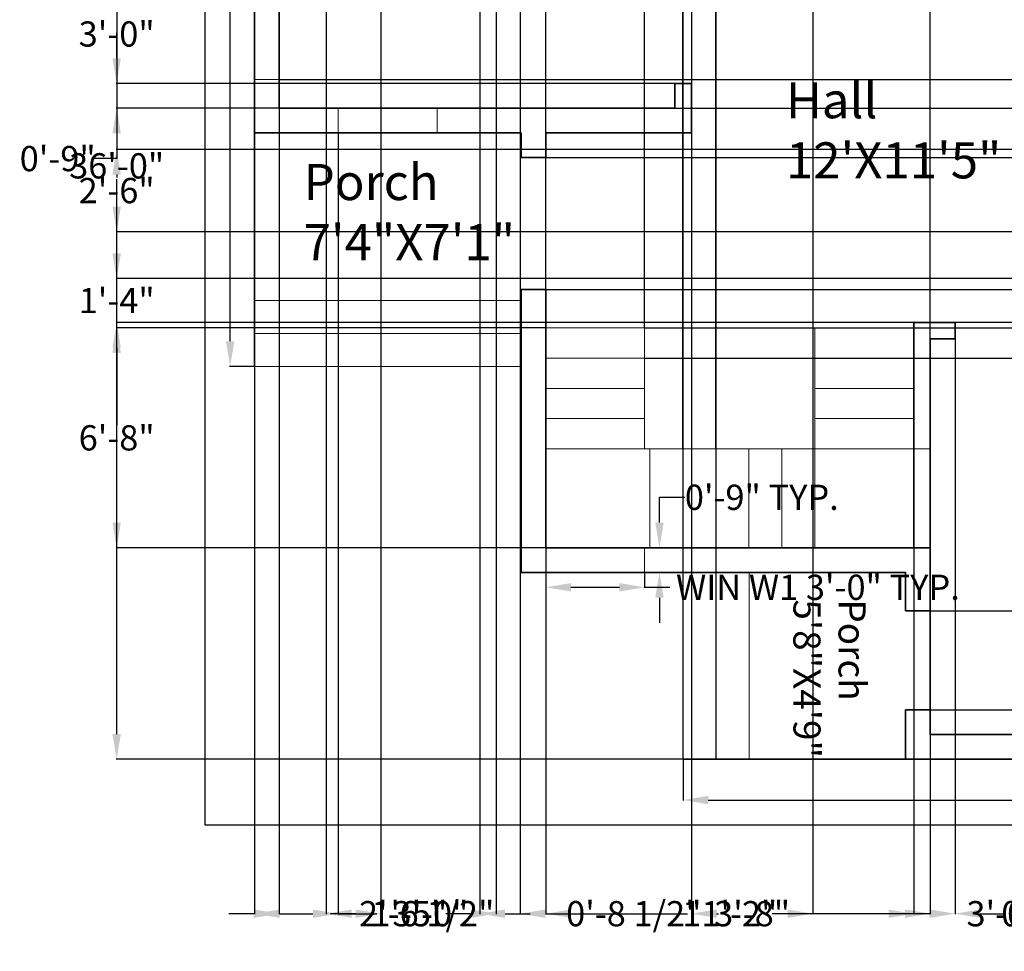
# Model space of a CAD drawing. Units: inches. Extents: x -69 to 558, y -494 to 191.
# Tile 1 of 3: x -69 to 289, y -494 to -155. Entities that reach past the tile are written whole.
import ezdxf

# ---------------------------------------------------------------- set-up
doc = ezdxf.new("R2010")
doc.units = ezdxf.units.IN
doc.header["$MEASUREMENT"] = 0
for name, color, linetype, lineweight in [('A-ANNO-DIMS', 2, 'Continuous', 18), ('A-AREA-IDEN', 7, 'Continuous', 18), ('A-FLOR-STRS', 3, 'Continuous', 18), ('A-GLAZ', 4, 'Continuous', 18), ('A-WALL', 7, 'Continuous', 35), ('C-PROP', 8, 'Continuous', 25)]:
    doc.layers.add(name, color=color, linetype=linetype, lineweight=lineweight)
doc.styles.get("Standard").update_dxf_attribs({"font": 'arial.ttf'})
doc.dimstyles.get("Standard").update_dxf_attribs({"dimtxt": 9.18, "dimasz": 9.18, "dimexe": 0.18, "dimexo": 0.0625, "dimgap": 0.09, "dimtad": 0, "dimtih": 1, "dimtoh": 1, "dimdec": 1, "dimzin": 0, "dimdsep": 46, "dimlunit": 3, "dimtxsty": 'Standard', "dimcen": 9, "dimadec": 0, "dimazin": 0, "dimtfac": 1, "dimtdec": 1, "dimtofl": 0, "dimtmove": 0, "dimatfit": 3, "dimfxl": 1, "dimtolj": 1, "dimtzin": 0, "dimarcsym": 0})

# ---------------------------------------------------------------- blocks, each defined once
blk = doc.blocks.new('*U1')
blk.add_line((-18, 0), (18, 0))
blk = doc.blocks.new('*U2')
at = {"layer": 'A-FLOR-STRS', "color": 0, "linetype": 'ByBlock', "lineweight": -2, "transparency": 16777216}
for p in [(0, 44), (0, 33), (0, 22), (0, 11), (0, 0)]:
    blk.add_blockref('*U1', p, dxfattribs=at)
blk = doc.blocks.new('*U3')
blk.add_line((0, -18), (0, 18))
blk = doc.blocks.new('*U4')
at = {"layer": 'A-FLOR-STRS', "color": 0, "linetype": 'ByBlock', "lineweight": -2, "transparency": 16777216}
for p in [(0, 0), (12, 0), (24, 0), (36, 0), (48, 0), (60, 0)]:
    blk.add_blockref('*U3', p, dxfattribs=at)
blk = doc.blocks.new('*U5')
blk.add_line((18, 0), (-18, 0))
blk = doc.blocks.new('*U6')
at = {"layer": 'A-FLOR-STRS', "color": 0, "linetype": 'ByBlock', "lineweight": -2, "transparency": 16777216}
for p in [(0, 44), (0, 33), (0, 22), (0, 11), (0, 0)]:
    blk.add_blockref('*U5', p, dxfattribs=at)
blk = doc.blocks.new('*D13')
at = {"layer": 'A-ANNO-DIMS', "color": 0, "lineweight": -2, "transparency": 16777216}
for p, q in [((16.29, 7.7), (7.29, 7.7)), ((7.47, -1.48), (7.47, -132.03)), ((7.47, -272.12), (7.47, -141.58)), ((16.29, -281.3), (7.29, -281.3))]:
    blk.add_line(p, q, dxfattribs=at)
at = {"layer": 'A-ANNO-DIMS', "color": 0, "transparency": 16777216}
for points in [[(5.94, -1.48), (9, -1.48), (7.47, 7.7)], [(5.94, -272.12), (9, -272.12), (7.47, -281.3)]]:
    blk.add_solid(points, dxfattribs=at)
at = {"layer": 'Defpoints', "color": 0, "transparency": 16777216}
for p in [(7.47, 7.7), (16.36, 7.7), (16.36, -281.3)]:
    blk.add_point(p, dxfattribs=at)
at = {"layer": 'A-ANNO-DIMS', "color": 0, "transparency": 16777216, "insert": (7.47, -136.8), "char_height": 9.18, "attachment_point": 5}
blk.add_mtext('\\A1;24\'-1.0"', dxfattribs=at)
blk = doc.blocks.new('*D14')
at = {"layer": 'A-ANNO-DIMS', "color": 0, "lineweight": -2, "transparency": 16777216}
for p, q in [((172.36, -424.37), (172.36, -439.31)), ((463.36, -424.37), (463.36, -439.31)), ((181.54, -439.13), (296.57, -439.13)), ((454.18, -439.13), (339.14, -439.13))]:
    blk.add_line(p, q, dxfattribs=at)
at = {"layer": 'A-ANNO-DIMS', "color": 0, "transparency": 16777216}
for points in [[(181.54, -437.6), (181.54, -440.66), (172.36, -439.13)], [(454.18, -437.6), (454.18, -440.66), (463.36, -439.13)]]:
    blk.add_solid(points, dxfattribs=at)
at = {"layer": 'Defpoints', "color": 0, "transparency": 16777216}
for p in [(172.36, -424.3), (463.36, -424.3), (172.36, -439.13)]:
    blk.add_point(p, dxfattribs=at)
at = {"layer": 'A-ANNO-DIMS', "color": 0, "transparency": 16777216, "insert": (317.86, -439.13), "char_height": 9.18, "attachment_point": 5}
blk.add_mtext('\\A1;24\'-3.0"', dxfattribs=at)
blk = doc.blocks.new('WIN-36IN')
blk.add_lwpolyline([(0, 0), (0, 9), (36, 9), (36, 0)], close=True)
blk = doc.blocks.new('*D18')
at = {"layer": 'A-ANNO-DIMS', "color": 0, "lineweight": -2, "transparency": 16777216}
for p, q in [((122.36, -356.37), (122.36, -361.88)), ((158.36, -356.37), (158.36, -361.88)), ((131.54, -361.7), (149.18, -361.7)), ((158.36, -361.7), (167.54, -361.7))]:
    blk.add_line(p, q, dxfattribs=at)
at = {"layer": 'A-ANNO-DIMS', "color": 0, "transparency": 16777216}
for points in [[(131.54, -360.17), (131.54, -363.23), (122.36, -361.7)], [(149.18, -360.17), (149.18, -363.23), (158.36, -361.7)]]:
    blk.add_solid(points, dxfattribs=at)
at = {"layer": 'Defpoints', "color": 0, "transparency": 16777216}
for p in [(122.36, -356.3), (158.36, -356.3), (158.36, -361.7)]:
    blk.add_point(p, dxfattribs=at)
at = {"layer": 'A-ANNO-DIMS', "color": 0, "transparency": 16777216, "insert": (221.44, -361.7), "char_height": 9.18, "attachment_point": 5}
blk.add_mtext('\\A1;WIN W1 3\'-0" TYP.', dxfattribs=at)
blk = doc.blocks.new('*D19')
at = {"layer": 'A-ANNO-DIMS', "color": 0, "lineweight": -2, "transparency": 16777216}
for p, q in [((163.76, -338.12), (163.76, -328.94)), ((163.76, -328.94), (172.94, -328.94)), ((158.42, -347.3), (163.94, -347.3)), ((158.42, -356.3), (163.94, -356.3)), ((163.76, -365.48), (163.76, -374.66))]:
    blk.add_line(p, q, dxfattribs=at)
at = {"layer": 'A-ANNO-DIMS', "color": 0, "transparency": 16777216}
for points in [[(162.23, -338.12), (165.29, -338.12), (163.76, -347.3)], [(162.23, -365.48), (165.29, -365.48), (163.76, -356.3)]]:
    blk.add_solid(points, dxfattribs=at)
at = {"layer": 'Defpoints', "color": 0, "transparency": 16777216}
for p in [(158.36, -347.3), (163.76, -347.3), (158.36, -356.3)]:
    blk.add_point(p, dxfattribs=at)
at = {"layer": 'A-ANNO-DIMS', "color": 0, "transparency": 16777216, "insert": (201.01, -328.94), "char_height": 9.18, "attachment_point": 5}
blk.add_mtext('\\A1;0\'-9" TYP.', dxfattribs=at)
blk = doc.blocks.new('*D25')
at = {"layer": 'A-ANNO-DIMS', "color": 0, "lineweight": -2, "transparency": 16777216}
for p, q in [((16.29, 7.7), (-34.02, 7.7)), ((-33.84, -1.48), (-33.84, -203.52)), ((-33.84, -415.12), (-33.84, -213.09)), ((172.29, -424.3), (-34.02, -424.3))]:
    blk.add_line(p, q, dxfattribs=at)
at = {"layer": 'A-ANNO-DIMS', "color": 0, "transparency": 16777216}
for points in [[(-35.37, -1.48), (-32.31, -1.48), (-33.84, 7.7)], [(-35.37, -415.12), (-32.31, -415.12), (-33.84, -424.3)]]:
    blk.add_solid(points, dxfattribs=at)
at = {"layer": 'Defpoints', "color": 0, "transparency": 16777216}
for p in [(16.36, 7.7), (-33.84, -424.3), (172.36, -424.3)]:
    blk.add_point(p, dxfattribs=at)
at = {"layer": 'A-ANNO-DIMS', "color": 0, "transparency": 16777216, "insert": (-33.84, -208.3), "char_height": 9.18, "attachment_point": 5}
blk.add_mtext('\\A1;36\'-0"', dxfattribs=at)
blk = doc.blocks.new('*D28')
at = {"layer": 'A-ANNO-DIMS', "color": 0, "lineweight": -2, "transparency": 16777216}
for p, q in [((122.36, -347.37), (122.36, -480.68)), ((256.36, -347.37), (256.36, -480.68)), ((131.54, -480.5), (173.93, -480.5)), ((247.18, -480.5), (204.78, -480.5))]:
    blk.add_line(p, q, dxfattribs=at)
at = {"layer": 'A-ANNO-DIMS', "color": 0, "transparency": 16777216}
for points in [[(131.54, -478.97), (131.54, -482.03), (122.36, -480.5)], [(247.18, -478.97), (247.18, -482.03), (256.36, -480.5)]]:
    blk.add_solid(points, dxfattribs=at)
at = {"layer": 'Defpoints', "color": 0, "transparency": 16777216}
for p in [(122.36, -347.3), (256.36, -347.3), (256.36, -480.5)]:
    blk.add_point(p, dxfattribs=at)
at = {"layer": 'A-ANNO-DIMS', "color": 0, "transparency": 16777216, "insert": (189.36, -480.5), "char_height": 9.18, "attachment_point": 5}
blk.add_mtext('\\A1;11\'-2"', dxfattribs=at)
blk = doc.blocks.new('*D29')
at = {"layer": 'A-ANNO-DIMS', "color": 0, "lineweight": -2, "transparency": 16777216}
for p, q in [((122.29, -267.3), (-34.02, -267.3)), ((-33.84, -276.48), (-33.84, -302.53)), ((-33.84, -338.12), (-33.84, -312.08)), ((122.29, -347.3), (-34.02, -347.3))]:
    blk.add_line(p, q, dxfattribs=at)
at = {"layer": 'A-ANNO-DIMS', "color": 0, "transparency": 16777216}
for points in [[(-35.37, -276.48), (-32.31, -276.48), (-33.84, -267.3)], [(-35.37, -338.12), (-32.31, -338.12), (-33.84, -347.3)]]:
    blk.add_solid(points, dxfattribs=at)
at = {"layer": 'Defpoints', "color": 0, "transparency": 16777216}
for p in [(122.36, -267.3), (-33.84, -347.3), (122.36, -347.3)]:
    blk.add_point(p, dxfattribs=at)
at = {"layer": 'A-ANNO-DIMS', "color": 0, "transparency": 16777216, "insert": (-33.84, -307.3), "char_height": 9.18, "attachment_point": 5}
blk.add_mtext('\\A1;6\'-8"', dxfattribs=at)
blk = doc.blocks.new('*D30')
at = {"layer": 'A-ANNO-DIMS', "color": 0, "lineweight": -2, "transparency": 16777216}
for p, q in [((113.177437, 63.89515), (103.997437, 63.89515)), ((122.357437, -267.24235), (122.357437, 64.07515)), ((158.357437, -267.24235), (158.357437, 64.07515)), ((167.537437, 63.89515), (176.717437, 63.89515))]:
    blk.add_line(p, q, dxfattribs=at)
at = {"layer": 'A-ANNO-DIMS', "color": 0, "transparency": 16777216}
for points in [[(113.177437, 65.42515), (113.177437, 62.36515), (122.357437, 63.89515)], [(167.537437, 65.42515), (167.537437, 62.36515), (158.357437, 63.89515)]]:
    blk.add_solid(points, dxfattribs=at)
at = {"layer": 'Defpoints', "color": 0, "transparency": 16777216}
for p in [(158.357437, 63.89515), (122.357437, -267.30485), (158.357437, -267.30485)]:
    blk.add_point(p, dxfattribs=at)
at = {"layer": 'A-ANNO-DIMS', "color": 0, "transparency": 16777216, "insert": (140.357437, 63.89515), "char_height": 9.18, "attachment_point": 5}
blk.add_mtext('\\A1;3\'-0"', dxfattribs=at)
blk = doc.blocks.new('*D31')
at = {"layer": 'A-ANNO-DIMS', "color": 0, "lineweight": -2, "transparency": 16777216}
for p, q in [((522.557437, -258.12485), (522.557437, -248.94485)), ((158.419937, -267.30485), (522.737437, -267.30485)), ((158.419937, -278.30485), (522.737437, -278.30485)), ((522.557437, -287.48485), (522.557437, -296.66485))]:
    blk.add_line(p, q, dxfattribs=at)
at = {"layer": 'A-ANNO-DIMS', "color": 0, "transparency": 16777216}
for points in [[(521.027437, -258.12485), (524.087437, -258.12485), (522.557437, -267.30485)], [(521.027437, -287.48485), (524.087437, -287.48485), (522.557437, -278.30485)]]:
    blk.add_solid(points, dxfattribs=at)
at = {"layer": 'Defpoints', "color": 0, "transparency": 16777216}
for p in [(158.357437, -267.30485), (158.357437, -278.30485), (522.557437, -278.30485)]:
    blk.add_point(p, dxfattribs=at)
at = {"layer": 'A-ANNO-DIMS', "color": 0, "transparency": 16777216, "insert": (522.557437, -272.80485), "char_height": 9.18, "attachment_point": 5}
blk.add_mtext('\\A1;0\'-11"', dxfattribs=at)
blk = doc.blocks.new('*D32')
at = {"layer": 'A-ANNO-DIMS', "color": 0, "lineweight": -2, "transparency": 16777216}
for p, q in [((163.09, 63.9), (153.91, 63.9)), ((172.27, -311.24), (172.27, 64.08)), ((184.27, -311.24), (184.27, 64.08)), ((193.45, 63.9), (202.63, 63.9))]:
    blk.add_line(p, q, dxfattribs=at)
at = {"layer": 'A-ANNO-DIMS', "color": 0, "transparency": 16777216}
for points in [[(163.09, 65.43), (163.09, 62.37), (172.27, 63.9)], [(193.45, 65.43), (193.45, 62.37), (184.27, 63.9)]]:
    blk.add_solid(points, dxfattribs=at)
at = {"layer": 'Defpoints', "color": 0, "transparency": 16777216}
for p in [(184.27, 63.9), (172.27, -311.3), (184.27, -311.3)]:
    blk.add_point(p, dxfattribs=at)
at = {"layer": 'A-ANNO-DIMS', "color": 0, "transparency": 16777216, "insert": (214.49, 63.9), "char_height": 9.18, "attachment_point": 5}
blk.add_mtext('\\A1;1\'-0"', dxfattribs=at)
blk = doc.blocks.new('*D37')
at = {"layer": 'A-ANNO-DIMS', "color": 0, "lineweight": -2, "transparency": 16777216}
for p, q in [((175.36, -1.37), (175.36, -480.68)), ((219.59, -1.37), (219.59, -480.68)), ((184.54, -480.5), (185.19, -480.5)), ((210.41, -480.5), (209.76, -480.5))]:
    blk.add_line(p, q, dxfattribs=at)
at = {"layer": 'A-ANNO-DIMS', "color": 0, "transparency": 16777216}
for points in [[(184.54, -478.97), (184.54, -482.03), (175.36, -480.5)], [(210.41, -478.97), (210.41, -482.03), (219.59, -480.5)]]:
    blk.add_solid(points, dxfattribs=at)
at = {"layer": 'Defpoints', "color": 0, "transparency": 16777216}
for p in [(175.36, -1.3), (219.59, -1.3), (219.59, -480.5)]:
    blk.add_point(p, dxfattribs=at)
at = {"layer": 'A-ANNO-DIMS', "color": 0, "transparency": 16777216, "insert": (197.48, -480.5), "char_height": 9.18, "attachment_point": 5}
blk.add_mtext('\\A1;3\'-8"', dxfattribs=at)
blk = doc.blocks.new('*D38')
at = {"layer": 'A-ANNO-DIMS', "color": 0, "lineweight": -2, "transparency": 16777216}
for p, q in [((-33.84, -240.17), (-33.84, -230.99)), ((454.29, -249.35), (-34.02, -249.35)), ((454.29, -265.3), (-34.02, -265.3)), ((-33.84, -274.48), (-33.84, -283.66))]:
    blk.add_line(p, q, dxfattribs=at)
at = {"layer": 'A-ANNO-DIMS', "color": 0, "transparency": 16777216}
for points in [[(-35.37, -240.17), (-32.31, -240.17), (-33.84, -249.35)], [(-35.37, -274.48), (-32.31, -274.48), (-33.84, -265.3)]]:
    blk.add_solid(points, dxfattribs=at)
at = {"layer": 'Defpoints', "color": 0, "transparency": 16777216}
for p in [(-33.84, -249.35), (454.36, -249.35), (454.36, -265.3)]:
    blk.add_point(p, dxfattribs=at)
at = {"layer": 'A-ANNO-DIMS', "color": 0, "transparency": 16777216, "insert": (-33.84, -257.33), "char_height": 9.18, "attachment_point": 5}
blk.add_mtext('\\A1;1\'-4"', dxfattribs=at)
blk = doc.blocks.new('*D39')
at = {"layer": 'A-ANNO-DIMS', "color": 0, "lineweight": -2, "transparency": 16777216}
for p, q in [((16.36, -196.37), (16.36, -480.68)), ((46.78, -196.37), (46.78, -480.68)), ((25.54, -480.5), (37.6, -480.5)), ((46.78, -480.5), (55.96, -480.5))]:
    blk.add_line(p, q, dxfattribs=at)
at = {"layer": 'A-ANNO-DIMS', "color": 0, "transparency": 16777216}
for points in [[(25.54, -478.97), (25.54, -482.03), (16.36, -480.5)], [(37.6, -478.97), (37.6, -482.03), (46.78, -480.5)]]:
    blk.add_solid(points, dxfattribs=at)
at = {"layer": 'Defpoints', "color": 0, "transparency": 16777216}
for p in [(16.36, -196.3), (46.78, -196.3), (46.78, -480.5)]:
    blk.add_point(p, dxfattribs=at)
at = {"layer": 'A-ANNO-DIMS', "color": 0, "transparency": 16777216, "insert": (79.02, -480.5), "char_height": 9.18, "attachment_point": 5}
blk.add_mtext('\\A1;2\'-6 1/2"', dxfattribs=at)
blk = doc.blocks.new('*D40')
at = {"layer": 'A-ANNO-DIMS', "color": 0, "lineweight": -2, "transparency": 16777216}
for p, q in [((25.36, -1.37), (25.36, -480.68)), ((42.48, -1.37), (42.48, -480.68)), ((16.18, -480.5), (7, -480.5)), ((51.66, -480.5), (60.84, -480.5))]:
    blk.add_line(p, q, dxfattribs=at)
at = {"layer": 'A-ANNO-DIMS', "color": 0, "transparency": 16777216}
for points in [[(16.18, -478.97), (16.18, -482.03), (25.36, -480.5)], [(51.66, -478.97), (51.66, -482.03), (42.48, -480.5)]]:
    blk.add_solid(points, dxfattribs=at)
at = {"layer": 'Defpoints', "color": 0, "transparency": 16777216}
for p in [(25.36, -1.3), (42.48, -1.3), (42.48, -480.5)]:
    blk.add_point(p, dxfattribs=at)
at = {"layer": 'A-ANNO-DIMS', "color": 0, "transparency": 16777216, "insert": (72.7, -480.5), "char_height": 9.18, "attachment_point": 5}
blk.add_mtext('\\A1;1\'-5"', dxfattribs=at)
blk = doc.blocks.new('*D41')
at = {"layer": 'A-ANNO-DIMS', "color": 0, "lineweight": -2, "transparency": 16777216}
for p, q in [((104.36, -1.37), (104.36, -480.68)), ((113.07, -1.37), (113.07, -480.68)), ((95.18, -480.5), (86, -480.5)), ((122.25, -480.5), (131.43, -480.5))]:
    blk.add_line(p, q, dxfattribs=at)
at = {"layer": 'A-ANNO-DIMS', "color": 0, "transparency": 16777216}
for points in [[(95.18, -478.97), (95.18, -482.03), (104.36, -480.5)], [(122.25, -478.97), (122.25, -482.03), (113.07, -480.5)]]:
    blk.add_solid(points, dxfattribs=at)
at = {"layer": 'Defpoints', "color": 0, "transparency": 16777216}
for p in [(104.36, -1.3), (113.07, -1.3), (113.07, -480.5)]:
    blk.add_point(p, dxfattribs=at)
at = {"layer": 'A-ANNO-DIMS', "color": 0, "transparency": 16777216, "insert": (154.42, -480.5), "char_height": 9.18, "attachment_point": 5}
blk.add_mtext('\\A1;0\'-8 1/2"', dxfattribs=at)
blk = doc.blocks.new('*D44')
at = {"layer": 'A-ANNO-DIMS', "color": 0, "lineweight": -2, "transparency": 16777216}
for p, q in [((522.557437, -167.693456), (522.557437, -158.513456)), ((25.419937, -176.873456), (522.737437, -176.873456)), ((25.419937, -187.30485), (522.737437, -187.30485)), ((522.557437, -196.48485), (522.557437, -205.66485))]:
    blk.add_line(p, q, dxfattribs=at)
at = {"layer": 'A-ANNO-DIMS', "color": 0, "transparency": 16777216}
for points in [[(521.027437, -167.693456), (524.087437, -167.693456), (522.557437, -176.873456)], [(521.027437, -196.48485), (524.087437, -196.48485), (522.557437, -187.30485)]]:
    blk.add_solid(points, dxfattribs=at)
at = {"layer": 'Defpoints', "color": 0, "transparency": 16777216}
for p in [(25.357437, -176.873456), (522.557437, -176.873456), (25.357437, -187.30485)]:
    blk.add_point(p, dxfattribs=at)
at = {"layer": 'A-ANNO-DIMS', "color": 0, "transparency": 16777216, "insert": (522.557437, -182.089153), "char_height": 9.18, "attachment_point": 5}
blk.add_mtext('\\A1;0\'-10 1/2"', dxfattribs=at)
blk = doc.blocks.new('*D47')
at = {"layer": 'A-ANNO-DIMS', "color": 0, "lineweight": -2, "transparency": 16777216}
for p, q in [((262.36, -415.24), (262.36, 64.08)), ((271.54, 63.9), (273.12, 63.9)), ((320.68, 63.9), (319.09, 63.9)), ((329.86, -415.24), (329.86, 64.08))]:
    blk.add_line(p, q, dxfattribs=at)
at = {"layer": 'A-ANNO-DIMS', "color": 0, "transparency": 16777216}
for points in [[(271.54, 65.43), (271.54, 62.37), (262.36, 63.9)], [(320.68, 65.43), (320.68, 62.37), (329.86, 63.9)]]:
    blk.add_solid(points, dxfattribs=at)
at = {"layer": 'Defpoints', "color": 0, "transparency": 16777216}
for p in [(329.86, 63.9), (262.36, -415.3), (329.86, -415.3)]:
    blk.add_point(p, dxfattribs=at)
at = {"layer": 'A-ANNO-DIMS', "color": 0, "transparency": 16777216, "insert": (296.11, 63.9), "char_height": 9.18, "attachment_point": 5}
blk.add_mtext('\\A1;5\'-7 1/2"', dxfattribs=at)
blk = doc.blocks.new('*D50')
at = {"layer": 'A-ANNO-DIMS', "color": 0, "lineweight": -2, "transparency": 16777216}
for p, q in [((169.29, -142.3), (-34.02, -142.3)), ((-33.84, -151.48), (-33.84, -155.52)), ((-33.84, -169.12), (-33.84, -165.09)), ((169.29, -178.3), (-34.02, -178.3))]:
    blk.add_line(p, q, dxfattribs=at)
at = {"layer": 'A-ANNO-DIMS', "color": 0, "transparency": 16777216}
for points in [[(-35.37, -151.48), (-32.31, -151.48), (-33.84, -142.3)], [(-35.37, -169.12), (-32.31, -169.12), (-33.84, -178.3)]]:
    blk.add_solid(points, dxfattribs=at)
at = {"layer": 'Defpoints', "color": 0, "transparency": 16777216}
for p in [(169.36, -142.3), (-33.84, -178.3), (169.36, -178.3)]:
    blk.add_point(p, dxfattribs=at)
at = {"layer": 'A-ANNO-DIMS', "color": 0, "transparency": 16777216, "insert": (-33.84, -160.3), "char_height": 9.18, "attachment_point": 5}
blk.add_mtext('\\A1;3\'-0"', dxfattribs=at)
blk = doc.blocks.new('*D51')
at = {"layer": 'A-ANNO-DIMS', "color": 0, "lineweight": -2, "transparency": 16777216}
for p, q in [((-33.84, -169.12), (-33.84, -159.94)), ((169.29, -178.3), (-34.02, -178.3)), ((169.29, -187.3), (-34.02, -187.3)), ((-33.84, -196.48), (-33.84, -205.66)), ((-33.84, -205.66), (-43.02, -205.66))]:
    blk.add_line(p, q, dxfattribs=at)
at = {"layer": 'A-ANNO-DIMS', "color": 0, "transparency": 16777216}
for points in [[(-35.37, -169.12), (-32.31, -169.12), (-33.84, -178.3)], [(-35.37, -196.48), (-32.31, -196.48), (-33.84, -187.3)]]:
    blk.add_solid(points, dxfattribs=at)
at = {"layer": 'Defpoints', "color": 0, "transparency": 16777216}
for p in [(169.36, -178.3), (-33.84, -187.3), (169.36, -187.3)]:
    blk.add_point(p, dxfattribs=at)
at = {"layer": 'A-ANNO-DIMS', "color": 0, "transparency": 16777216, "insert": (-55.31, -205.66), "char_height": 9.18, "attachment_point": 5}
blk.add_mtext('\\A1;0\'-9"', dxfattribs=at)
blk = doc.blocks.new('*D52')
at = {"layer": 'A-ANNO-DIMS', "color": 0, "lineweight": -2, "transparency": 16777216}
for p, q in [((271.357437, -271.36735), (271.357437, -480.68485)), ((307.357437, -271.36735), (307.357437, -480.68485)), ((262.177437, -480.50485), (252.997437, -480.50485)), ((316.537437, -480.50485), (325.717437, -480.50485))]:
    blk.add_line(p, q, dxfattribs=at)
at = {"layer": 'A-ANNO-DIMS', "color": 0, "transparency": 16777216}
for points in [[(262.177437, -478.97485), (262.177437, -482.03485), (271.357437, -480.50485)], [(316.537437, -478.97485), (316.537437, -482.03485), (307.357437, -480.50485)]]:
    blk.add_solid(points, dxfattribs=at)
at = {"layer": 'Defpoints', "color": 0, "transparency": 16777216}
for p in [(271.357437, -271.30485), (307.357437, -271.30485), (307.357437, -480.50485)]:
    blk.add_point(p, dxfattribs=at)
at = {"layer": 'A-ANNO-DIMS', "color": 0, "transparency": 16777216, "insert": (289.357437, -480.50485), "char_height": 9.18, "attachment_point": 5}
blk.add_mtext('\\A1;3\'-0"', dxfattribs=at)
blk = doc.blocks.new('*D53')
at = {"layer": 'A-ANNO-DIMS', "color": 0, "lineweight": -2, "transparency": 16777216}
for p, q in [((262.36, -271.37), (262.36, -480.68)), ((271.36, -271.37), (271.36, -480.68)), ((253.18, -480.5), (244, -480.5)), ((280.54, -480.5), (289.72, -480.5))]:
    blk.add_line(p, q, dxfattribs=at)
at = {"layer": 'A-ANNO-DIMS', "color": 0, "transparency": 16777216}
for points in [[(253.18, -478.97), (253.18, -482.03), (262.36, -480.5)], [(280.54, -478.97), (280.54, -482.03), (271.36, -480.5)]]:
    blk.add_solid(points, dxfattribs=at)
at = {"layer": 'Defpoints', "color": 0, "transparency": 16777216}
for p in [(262.36, -271.3), (271.36, -271.3), (271.36, -480.5)]:
    blk.add_point(p, dxfattribs=at)
at = {"layer": 'A-ANNO-DIMS', "color": 0, "transparency": 16777216, "insert": (302.01, -480.5), "char_height": 9.18, "attachment_point": 5}
blk.add_mtext('\\A1;0\'-9"', dxfattribs=at)
blk = doc.blocks.new('*D54')
at = {"layer": 'A-ANNO-DIMS', "color": 0, "lineweight": -2, "transparency": 16777216}
for p, q in [((358.29, -202.3), (-34.02, -202.3)), ((-33.84, -211.48), (-33.84, -212.53)), ((-33.84, -223.12), (-33.84, -222.08)), ((358.29, -232.3), (-34.02, -232.3))]:
    blk.add_line(p, q, dxfattribs=at)
at = {"layer": 'A-ANNO-DIMS', "color": 0, "transparency": 16777216}
for points in [[(-35.37, -211.48), (-32.31, -211.48), (-33.84, -202.3)], [(-35.37, -223.12), (-32.31, -223.12), (-33.84, -232.3)]]:
    blk.add_solid(points, dxfattribs=at)
at = {"layer": 'Defpoints', "color": 0, "transparency": 16777216}
for p in [(358.36, -202.3), (-33.84, -232.3), (358.36, -232.3)]:
    blk.add_point(p, dxfattribs=at)
at = {"layer": 'A-ANNO-DIMS', "color": 0, "transparency": 16777216, "insert": (-33.84, -217.3), "char_height": 9.18, "attachment_point": 5}
blk.add_mtext('\\A1;2\'-6"', dxfattribs=at)
blk = doc.blocks.new('*D55')
at = {"layer": 'A-ANNO-DIMS', "color": 0, "lineweight": -2, "transparency": 16777216}
for p, q in [((262.42, -370.3), (522.74, -370.3)), ((522.56, -379.48), (522.56, -383.52)), ((522.56, -397.12), (522.56, -393.09)), ((262.42, -406.3), (522.74, -406.3))]:
    blk.add_line(p, q, dxfattribs=at)
at = {"layer": 'A-ANNO-DIMS', "color": 0, "transparency": 16777216}
for points in [[(521.03, -379.48), (524.09, -379.48), (522.56, -370.3)], [(521.03, -397.12), (524.09, -397.12), (522.56, -406.3)]]:
    blk.add_solid(points, dxfattribs=at)
at = {"layer": 'Defpoints', "color": 0, "transparency": 16777216}
for p in [(262.36, -370.3), (262.36, -406.3), (522.56, -406.3)]:
    blk.add_point(p, dxfattribs=at)
at = {"layer": 'A-ANNO-DIMS', "color": 0, "transparency": 16777216, "insert": (522.56, -388.3), "char_height": 9.18, "attachment_point": 5}
blk.add_mtext('\\A1;3\'-0"', dxfattribs=at)
blk = doc.blocks.new('*D56')
at = {"layer": 'A-ANNO-DIMS', "color": 0, "lineweight": -2, "transparency": 16777216}
for p, q in [((62.357437, -67.36735), (62.357437, -480.68485)), ((98.357437, -67.36735), (98.357437, -480.68485)), ((53.177437, -480.50485), (43.997437, -480.50485)), ((107.537437, -480.50485), (116.717437, -480.50485))]:
    blk.add_line(p, q, dxfattribs=at)
at = {"layer": 'A-ANNO-DIMS', "color": 0, "transparency": 16777216}
for points in [[(53.177437, -478.97485), (53.177437, -482.03485), (62.357437, -480.50485)], [(107.537437, -478.97485), (107.537437, -482.03485), (98.357437, -480.50485)]]:
    blk.add_solid(points, dxfattribs=at)
at = {"layer": 'Defpoints', "color": 0, "transparency": 16777216}
for p in [(62.357437, -67.30485), (98.357437, -67.30485), (98.357437, -480.50485)]:
    blk.add_point(p, dxfattribs=at)
at = {"layer": 'A-ANNO-DIMS', "color": 0, "transparency": 16777216, "insert": (80.357437, -480.50485), "char_height": 9.18, "attachment_point": 5}
blk.add_mtext('\\A1;3\'-0"', dxfattribs=at)
blk = doc.blocks.new('*D60')
at = {"layer": 'A-ANNO-DIMS', "color": 0, "lineweight": -2, "transparency": 16777216}
for p, q in [((122.42, -205.3), (522.74, -205.3)), ((522.56, -214.48), (522.56, -224.53)), ((522.56, -244.12), (522.56, -234.08)), ((122.42, -253.3), (522.74, -253.3))]:
    blk.add_line(p, q, dxfattribs=at)
at = {"layer": 'A-ANNO-DIMS', "color": 0, "transparency": 16777216}
for points in [[(521.03, -214.48), (524.09, -214.48), (522.56, -205.3)], [(521.03, -244.12), (524.09, -244.12), (522.56, -253.3)]]:
    blk.add_solid(points, dxfattribs=at)
at = {"layer": 'Defpoints', "color": 0, "transparency": 16777216}
for p in [(122.36, -205.3), (122.36, -253.3), (522.56, -253.3)]:
    blk.add_point(p, dxfattribs=at)
at = {"layer": 'A-ANNO-DIMS', "color": 0, "transparency": 16777216, "insert": (522.56, -229.3), "char_height": 9.18, "attachment_point": 5}
blk.add_mtext('\\A1;4\'-0"', dxfattribs=at)
blk = doc.blocks.new('*D61')
at = {"layer": 'A-ANNO-DIMS', "color": 0, "lineweight": -2, "transparency": 16777216}
for p, q in [((163.18, 63.9), (154, 63.9)), ((172.36, -424.24), (172.36, 64.08)), ((184.36, -424.24), (184.36, 64.08)), ((193.54, 63.9), (202.72, 63.9))]:
    blk.add_line(p, q, dxfattribs=at)
at = {"layer": 'A-ANNO-DIMS', "color": 0, "transparency": 16777216}
for points in [[(163.18, 65.43), (163.18, 62.37), (172.36, 63.9)], [(193.54, 65.43), (193.54, 62.37), (184.36, 63.9)]]:
    blk.add_solid(points, dxfattribs=at)
at = {"layer": 'Defpoints', "color": 0, "transparency": 16777216}
for p in [(184.36, 63.9), (172.36, -424.3), (184.36, -424.3)]:
    blk.add_point(p, dxfattribs=at)
at = {"layer": 'A-ANNO-DIMS', "color": 0, "transparency": 16777216, "insert": (214.58, 63.9), "char_height": 9.18, "attachment_point": 5}
blk.add_mtext('\\A1;1\'-0"', dxfattribs=at)

msp = doc.modelspace()

# ---------------------------------------------------------------- linework, layer by layer
at = {"layer": 'A-FLOR-STRS'}
for p, q in [((16.36, -257.3), (113.36, -257.3)), ((158.36, -311.3), (158.36, -267.3)), ((220.36, -311.3), (220.36, -267.3)), ((16.36, -269.3), (113.36, -269.3)), ((16.36, -281.3), (113.36, -281.3)), ((262.36, -311.3), (158.36, -311.3)), ((172.36, -424.3), (172.36, -356.3)), ((184.36, -424.3), (184.36, -356.3)), ((196.36, -424.3), (196.36, -356.3))]:
    msp.add_line(p, q, dxfattribs=at)
at = {"layer": 'A-WALL'}
for p, q in [((16.36, -281.3), (16.36, 7.7)), ((25.36, -187.3), (25.36, -67.3)), ((169.36, -187.3), (169.36, -178.3)), ((169.36, -178.3), (175.36, -178.3)), ((175.36, -196.3), (175.36, -178.3)), ((25.36, -187.3), (169.36, -187.3)), ((16.36, -196.3), (113.36, -196.3)), ((113.36, -205.3), (113.36, -196.3)), ((122.36, -205.3), (122.36, -196.3)), ((122.36, -196.3), (175.36, -196.3)), ((113.36, -205.3), (122.36, -205.3)), ((113.36, -356.3), (113.36, -253.3)), ((113.36, -253.3), (122.36, -253.3)), ((122.36, -347.3), (122.36, -253.3)), ((256.36, -347.3), (256.36, -265.3)), ((256.36, -265.3), (271.36, -265.3)), ((271.36, -271.3), (271.36, -265.3)), ((262.36, -271.3), (271.36, -271.3)), ((262.36, -370.3), (262.36, -271.3)), ((262.36, -347.3), (122.36, -347.3)), ((253.36, -356.3), (113.36, -356.3)), ((253.36, -370.3), (253.36, -356.3)), ((262.36, -370.3), (253.36, -370.3)), ((253.36, -424.3), (253.36, -406.3)), ((262.36, -406.3), (253.36, -406.3)), ((262.36, -415.3), (262.36, -406.3)), ((454.36, -415.3), (262.36, -415.3)), ((463.36, -424.3), (172.36, -424.3))]:
    msp.add_line(p, q, dxfattribs=at)
at = {"layer": 'C-PROP'}
for p, q in [((-1.64, -448.3), (-1.64, 31.7)), ((490.36, -448.3), (-1.64, -448.3))]:
    msp.add_line(p, q, dxfattribs=at)

# ---------------------------------------------------------------- block references
at = {"layer": 'A-FLOR-STRS'}
for name, p in [('*U6', (140.36, -311.3)), ('*U2', (238.36, -311.3)), ('*U4', (160.27, -329.3))]:
    msp.add_blockref(name, p, dxfattribs=at)
at = {"layer": 'A-GLAZ', "rotation": 270}
msp.add_blockref('WIN-36IN', (16.36, -140.87), dxfattribs=at)
at = {"layer": 'A-GLAZ'}
for p in [(46.78, -196.3), (122.36, -356.3)]:
    msp.add_blockref('WIN-36IN', p, dxfattribs=at)

# ---------------------------------------------------------------- texts
at = {"layer": 'A-AREA-IDEN', "char_height": 13.129, "attachment_point": 1}
for s, insert in [('Hall\\P12\'X11\'5"', (209.81, -177.85)), ('Porch\\P7\'4"X7\'1"', (34.22, -207.63))]:
    msp.add_mtext_dynamic_manual_height_columns(s, width=125.4475, gutter_width=65.65, heights=[60.44], dxfattribs=dict(at, insert=insert))
at = {"layer": 'A-AREA-IDEN', "insert": (238.8, -366.1), "char_height": 9.847, "attachment_point": 1, "rotation": 270}
msp.add_mtext_dynamic_manual_height_columns('Porch\\P5\'8"X4\'9"', width=94.0856, gutter_width=49.23, heights=[45.33], dxfattribs=at)

# ---------------------------------------------------------------- dimensions: what is measured, and where the dimension line sits
at = {"layer": 'A-ANNO-DIMS'}
for base, p1, p2, override, picture, middle in [((329.86, 63.9), (262.36, -415.3), (329.86, -415.3), {"dimdec": 1, "dimlfac": 1, "dimrnd": 0, "dimzin": 1, "dimdsep": 46, "dimlunit": 4, "dimfrac": 2}, '*D47', (296.11, 63.9)), ((158.36, 63.9), (122.36, -267.3), (158.36, -267.3), {"dimdec": 1, "dimlfac": 1, "dimrnd": 0, "dimzin": 1, "dimdsep": 46, "dimlunit": 4, "dimfrac": 2}, '*D30', (140.36, 63.9)), ((184.27, 63.9), (172.27, -311.3), (184.27, -311.3), {"dimdec": 1, "dimlfac": 1, "dimrnd": 0, "dimzin": 1, "dimdsep": 46, "dimlunit": 4, "dimfrac": 2}, '*D32', (214.49, 63.9)), ((184.36, 63.9), (172.36, -424.3), (184.36, -424.3), {"dimdec": 1, "dimlfac": 1, "dimrnd": 0, "dimzin": 1, "dimdsep": 46, "dimlunit": 4, "dimfrac": 2}, '*D61', (214.58, 63.9)), ((42.48, -480.5), (25.36, -1.3), (42.48, -1.3), {"dimdec": 1, "dimlfac": 1, "dimrnd": 0, "dimzin": 1, "dimdsep": 46, "dimlunit": 4, "dimfrac": 2}, '*D40', (72.7, -480.5)), ((113.07, -480.5), (104.36, -1.3), (113.07, -1.3), {"dimdec": 1, "dimlfac": 1, "dimrnd": 0, "dimzin": 1, "dimdsep": 46, "dimlunit": 4, "dimfrac": 2}, '*D41', (154.42, -480.5)), ((219.59, -480.5), (175.36, -1.3), (219.59, -1.3), {"dimdec": 1, "dimlfac": 1, "dimrnd": 0, "dimzin": 1, "dimdsep": 46, "dimlunit": 4, "dimfrac": 2}, '*D37', (197.48, -480.5)), ((98.36, -480.5), (62.36, -67.3), (98.36, -67.3), {"dimdec": 1, "dimlfac": 1, "dimrnd": 0, "dimzin": 1, "dimdsep": 46, "dimlunit": 4, "dimfrac": 2}, '*D56', (80.36, -480.5)), ((46.78, -480.5), (16.36, -196.3), (46.78, -196.3), {"dimdec": 1, "dimlfac": 1, "dimrnd": 0, "dimzin": 1, "dimdsep": 46, "dimlunit": 4, "dimfrac": 2}, '*D39', (79.02, -480.5)), ((271.36, -480.5), (262.36, -271.3), (271.36, -271.3), {"dimdec": 1, "dimlfac": 1, "dimrnd": 0, "dimzin": 1, "dimdsep": 46, "dimlunit": 4, "dimfrac": 2}, '*D53', (302.01, -480.5)), ((307.36, -480.5), (271.36, -271.3), (307.36, -271.3), {"dimdec": 1, "dimlfac": 1, "dimrnd": 0, "dimzin": 1, "dimdsep": 46, "dimlunit": 4, "dimfrac": 2}, '*D52', (289.36, -480.5)), ((256.36, -480.5), (122.36, -347.3), (256.36, -347.3), {"dimdec": 1, "dimlfac": 1, "dimrnd": 0, "dimzin": 1, "dimdsep": 46, "dimlunit": 4, "dimfrac": 2}, '*D28', (189.36, -480.5)), ((172.36, -439.13), (463.36, -424.3), (172.36, -424.3), {"dimclrd": 0, "dimclre": 0, "dimclrt": 0}, '*D14', (317.86, -439.13))]:
    dim = msp.add_linear_dim(base=base, p1=p1, p2=p2, dimstyle='Standard', override=override, dxfattribs=at)
    dim.commit()
    dim.dimension.update_dxf_attribs({"geometry": picture, "text_midpoint": middle})
for base, p1, p2, override, picture, middle in [((-33.84, -424.3), (16.36, 7.7), (172.36, -424.3), {"dimdec": 1, "dimlfac": 1, "dimrnd": 0, "dimzin": 1, "dimdsep": 46, "dimlunit": 4, "dimfrac": 2}, '*D25', (-33.84, -208.3)), ((7.47, 7.7), (16.36, -281.3), (16.36, 7.7), {"dimclrd": 0, "dimclre": 0, "dimclrt": 0}, '*D13', (7.47, -136.8)), ((-33.84, -178.3), (169.36, -142.3), (169.36, -178.3), {"dimdec": 1, "dimlfac": 1, "dimrnd": 0, "dimzin": 1, "dimdsep": 46, "dimlunit": 4, "dimfrac": 2}, '*D50', (-33.84, -160.3)), ((-33.84, -187.3), (169.36, -178.3), (169.36, -187.3), {"dimdec": 1, "dimlfac": 1, "dimrnd": 0, "dimzin": 1, "dimdsep": 46, "dimlunit": 4, "dimfrac": 2}, '*D51', (-55.31, -205.66)), ((522.56, -176.87), (25.36, -187.3), (25.36, -176.87), {"dimdec": 1, "dimlfac": 1, "dimrnd": 0, "dimzin": 1, "dimdsep": 46, "dimlunit": 4, "dimfrac": 2}, '*D44', (522.56, -182.09)), ((-33.84, -232.3), (358.36, -202.3), (358.36, -232.3), {"dimdec": 1, "dimlfac": 1, "dimrnd": 0, "dimzin": 1, "dimdsep": 46, "dimlunit": 4, "dimfrac": 2}, '*D54', (-33.84, -217.3)), ((522.56, -253.3), (122.36, -205.3), (122.36, -253.3), {"dimdec": 1, "dimlfac": 1, "dimrnd": 0, "dimzin": 1, "dimdsep": 46, "dimlunit": 4, "dimfrac": 2}, '*D60', (522.56, -229.3)), ((-33.8426, -249.3471), (454.3574, -265.3048), (454.3574, -249.3471), {"dimdec": 1, "dimlfac": 1, "dimrnd": 0, "dimzin": 1, "dimdsep": 46, "dimlunit": 4, "dimfrac": 2}, '*D38', (-33.8426, -257.326)), ((522.56, -278.3), (158.36, -267.3), (158.36, -278.3), {"dimdec": 1, "dimlfac": 1, "dimrnd": 0, "dimzin": 1, "dimdsep": 46, "dimlunit": 4, "dimfrac": 2}, '*D31', (522.56, -272.8)), ((-33.84, -347.3), (122.36, -267.3), (122.36, -347.3), {"dimdec": 1, "dimlfac": 1, "dimrnd": 0, "dimzin": 1, "dimdsep": 46, "dimlunit": 4, "dimfrac": 2}, '*D29', (-33.84, -307.3)), ((522.56, -406.3), (262.36, -370.3), (262.36, -406.3), {"dimdec": 1, "dimlfac": 1, "dimrnd": 0, "dimzin": 1, "dimdsep": 46, "dimlunit": 4, "dimfrac": 2}, '*D55', (522.56, -388.3))]:
    dim = msp.add_linear_dim(base=base, p1=p1, p2=p2, angle=90, dimstyle='Standard', override=override, dxfattribs=at)
    dim.commit()
    dim.dimension.update_dxf_attribs({"geometry": picture, "text_midpoint": middle})
dim = msp.add_linear_dim(base=(163.76, -347.3), p1=(158.36, -356.3), p2=(158.36, -347.3), angle=90, text='<> TYP.', dimstyle='Standard', override={"dimdec": 1, "dimlfac": 1, "dimrnd": 0, "dimzin": 1, "dimdsep": 46, "dimlunit": 4, "dimfrac": 2}, dxfattribs=at)
dim.commit()
dim.dimension.update_dxf_attribs({"geometry": '*D19', "text_midpoint": (201.01, -328.94)})
dim = msp.add_linear_dim(base=(158.36, -361.7), p1=(122.36, -356.3), p2=(158.36, -356.3), text='WIN W1 <> TYP.', dimstyle='Standard', override={"dimdec": 1, "dimlfac": 1, "dimrnd": 0, "dimzin": 1, "dimdsep": 46, "dimlunit": 4, "dimfrac": 2}, dxfattribs=at)
dim.commit()
dim.dimension.update_dxf_attribs({"geometry": '*D18', "text_midpoint": (221.44, -361.7)})

doc.saveas('drawing.dxf')
